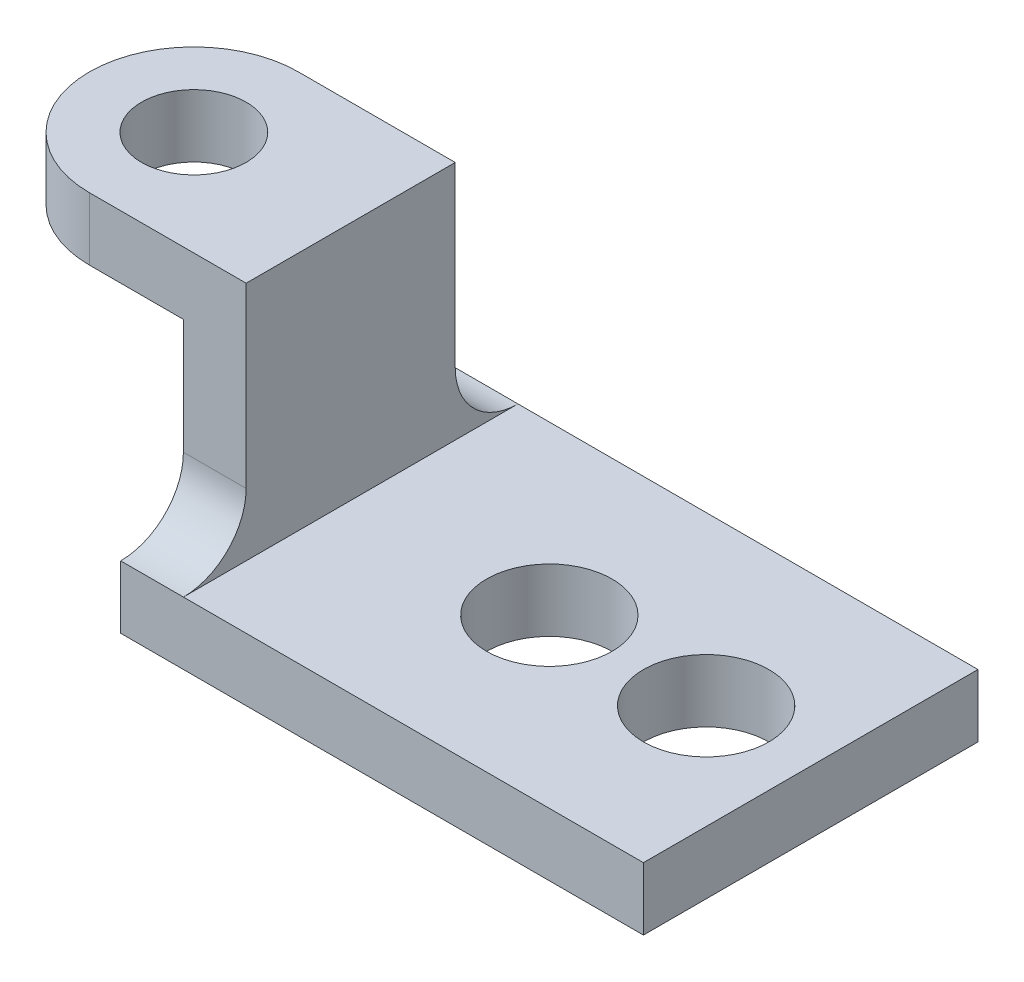
ISO-10303-21;
HEADER;
FILE_DESCRIPTION(('STEP AP214'),'2;1');
FILE_NAME('part.step','',(''),(''),'','','');
FILE_SCHEMA(('AUTOMOTIVE_DESIGN { 1 0 10303 214 1 1 1 1 }'));
ENDSEC;
DATA;
#1=APPLICATION_CONTEXT('core data for automotive mechanical design processes');
#2=APPLICATION_PROTOCOL_DEFINITION('international standard','automotive_design',2000,#1);
#3=PRODUCT_CONTEXT('',#1,'mechanical');
#4=PRODUCT('Part','Part','',(#3));
#5=PRODUCT_RELATED_PRODUCT_CATEGORY('part','',(#4));
#6=PRODUCT_DEFINITION_FORMATION('','',#4);
#7=PRODUCT_DEFINITION_CONTEXT('part definition',#1,'design');
#8=PRODUCT_DEFINITION('design','',#6,#7);
#9=PRODUCT_DEFINITION_SHAPE('','',#8);
#10=(LENGTH_UNIT() NAMED_UNIT(*) SI_UNIT(.MILLI.,.METRE.));
#11=(NAMED_UNIT(*) PLANE_ANGLE_UNIT() SI_UNIT($,.RADIAN.));
#12=(NAMED_UNIT(*) SI_UNIT($,.STERADIAN.) SOLID_ANGLE_UNIT());
#13=UNCERTAINTY_MEASURE_WITH_UNIT(LENGTH_MEASURE(1.E-05),#10,'distance_accuracy_value','');
#14=(GEOMETRIC_REPRESENTATION_CONTEXT(3) GLOBAL_UNCERTAINTY_ASSIGNED_CONTEXT((#13)) GLOBAL_UNIT_ASSIGNED_CONTEXT((#10,
#11,#12)) REPRESENTATION_CONTEXT('',''));
#15=CARTESIAN_POINT('',(0.,0.,0.));
#16=DIRECTION('',(0.,0.,1.));
#17=DIRECTION('',(1.,0.,0.));
#18=AXIS2_PLACEMENT_3D('',#15,#16,#17);
#19=CARTESIAN_POINT('',(-50.,12.,32.));
#20=DIRECTION('',(1.,0.,0.));
#21=DIRECTION('',(0.,0.,-1.));
#22=AXIS2_PLACEMENT_3D('',#19,#20,#21);
#23=PLANE('',#22);
#24=DIRECTION('',(0.,0.,1.));
#25=VECTOR('',#24,1.);
#26=CARTESIAN_POINT('',(-50.,46.,32.));
#27=LINE('',#26,#25);
#28=CARTESIAN_POINT('',(-50.,46.,-20.));
#29=VERTEX_POINT('',#28);
#30=CARTESIAN_POINT('',(-50.,46.,20.));
#31=VERTEX_POINT('',#30);
#32=EDGE_CURVE('E154',#29,#31,#27,.T.);
#33=ORIENTED_EDGE('',*,*,#32,.F.);
#34=DIRECTION('',(0.,-1.,0.));
#35=VECTOR('',#34,1.);
#36=CARTESIAN_POINT('',(-50.,58.,-20.));
#37=LINE('',#36,#35);
#38=CARTESIAN_POINT('',(-50.,24.,-20.));
#39=VERTEX_POINT('',#38);
#40=EDGE_CURVE('E133',#29,#39,#37,.T.);
#41=ORIENTED_EDGE('',*,*,#40,.T.);
#42=CARTESIAN_POINT('',(-50.,24.,-32.));
#43=DIRECTION('',(1.,0.,0.));
#44=DIRECTION('',(0.,0.,-1.));
#45=AXIS2_PLACEMENT_3D('',#42,#43,#44);
#46=CIRCLE('',#45,12.);
#47=CARTESIAN_POINT('',(-50.,12.,-32.));
#48=VERTEX_POINT('',#47);
#49=EDGE_CURVE('E222',#39,#48,#46,.T.);
#50=ORIENTED_EDGE('',*,*,#49,.T.);
#51=DIRECTION('',(0.,-1.,0.));
#52=VECTOR('',#51,1.);
#53=CARTESIAN_POINT('',(-50.,12.,-32.));
#54=LINE('',#53,#52);
#55=CARTESIAN_POINT('',(-50.,0.,-32.));
#56=VERTEX_POINT('',#55);
#57=EDGE_CURVE('E211',#48,#56,#54,.T.);
#58=ORIENTED_EDGE('',*,*,#57,.T.);
#59=DIRECTION('',(0.,0.,1.));
#60=VECTOR('',#59,1.);
#61=CARTESIAN_POINT('',(-50.,0.,32.));
#62=LINE('',#61,#60);
#63=CARTESIAN_POINT('',(-50.,0.,32.));
#64=VERTEX_POINT('',#63);
#65=EDGE_CURVE('E201',#56,#64,#62,.T.);
#66=ORIENTED_EDGE('',*,*,#65,.T.);
#67=DIRECTION('',(0.,-1.,0.));
#68=VECTOR('',#67,1.);
#69=CARTESIAN_POINT('',(-50.,12.,32.));
#70=LINE('',#69,#68);
#71=CARTESIAN_POINT('',(-50.,12.,32.));
#72=VERTEX_POINT('',#71);
#73=EDGE_CURVE('E208',#72,#64,#70,.T.);
#74=ORIENTED_EDGE('',*,*,#73,.F.);
#75=CARTESIAN_POINT('',(-50.,24.,32.));
#76=DIRECTION('',(1.,0.,0.));
#77=DIRECTION('',(0.,0.,-1.));
#78=AXIS2_PLACEMENT_3D('',#75,#76,#77);
#79=CIRCLE('',#78,12.);
#80=CARTESIAN_POINT('',(-50.,24.,20.));
#81=VERTEX_POINT('',#80);
#82=EDGE_CURVE('E11',#72,#81,#79,.T.);
#83=ORIENTED_EDGE('',*,*,#82,.T.);
#84=DIRECTION('',(0.,-1.,0.));
#85=VECTOR('',#84,1.);
#86=CARTESIAN_POINT('',(-50.,58.,20.));
#87=LINE('',#86,#85);
#88=EDGE_CURVE('E175',#31,#81,#87,.T.);
#89=ORIENTED_EDGE('',*,*,#88,.F.);
#90=EDGE_LOOP('',(#33,#41,#50,#58,#66,#74,#83,#89));
#91=FACE_BOUND('',#90,.T.);
#92=ADVANCED_FACE('F39',(#91),#23,.F.);
#93=CARTESIAN_POINT('',(0.,12.,0.));
#94=DIRECTION('',(0.,-1.,0.));
#95=DIRECTION('',(0.,0.,-1.));
#96=AXIS2_PLACEMENT_3D('',#93,#94,#95);
#97=PLANE('',#96);
#98=CARTESIAN_POINT('',(0.,12.,0.));
#99=DIRECTION('',(0.,1.,0.));
#100=DIRECTION('',(0.,0.,1.));
#101=AXIS2_PLACEMENT_3D('',#98,#99,#100);
#102=CIRCLE('',#101,12.);
#103=CARTESIAN_POINT('',(0.,12.,12.));
#104=VERTEX_POINT('',#103);
#105=EDGE_CURVE('E172',#104,#104,#102,.T.);
#106=ORIENTED_EDGE('',*,*,#105,.F.);
#107=EDGE_LOOP('',(#106));
#108=FACE_BOUND('',#107,.T.);
#109=CARTESIAN_POINT('',(30.,12.,0.));
#110=DIRECTION('',(0.,1.,0.));
#111=DIRECTION('',(0.,0.,1.));
#112=AXIS2_PLACEMENT_3D('',#109,#110,#111);
#113=CIRCLE('',#112,12.);
#114=CARTESIAN_POINT('',(30.,12.,12.));
#115=VERTEX_POINT('',#114);
#116=EDGE_CURVE('E182',#115,#115,#113,.T.);
#117=ORIENTED_EDGE('',*,*,#116,.F.);
#118=EDGE_LOOP('',(#117));
#119=FACE_BOUND('',#118,.T.);
#120=DIRECTION('',(-1.,0.,0.));
#121=VECTOR('',#120,1.);
#122=CARTESIAN_POINT('',(-50.,12.,-32.));
#123=LINE('',#122,#121);
#124=CARTESIAN_POINT('',(50.,12.,-32.));
#125=VERTEX_POINT('',#124);
#126=CARTESIAN_POINT('',(-38.,12.,-32.));
#127=VERTEX_POINT('',#126);
#128=EDGE_CURVE('E194',#125,#127,#123,.T.);
#129=ORIENTED_EDGE('',*,*,#128,.T.);
#130=DIRECTION('',(0.,0.,-1.));
#131=VECTOR('',#130,1.);
#132=CARTESIAN_POINT('',(-38.,12.,-20.));
#133=LINE('',#132,#131);
#134=CARTESIAN_POINT('',(-38.,12.,32.));
#135=VERTEX_POINT('',#134);
#136=EDGE_CURVE('E158',#135,#127,#133,.T.);
#137=ORIENTED_EDGE('',*,*,#136,.F.);
#138=DIRECTION('',(1.,0.,0.));
#139=VECTOR('',#138,1.);
#140=CARTESIAN_POINT('',(-50.,12.,32.));
#141=LINE('',#140,#139);
#142=CARTESIAN_POINT('',(50.,12.,32.));
#143=VERTEX_POINT('',#142);
#144=EDGE_CURVE('E193',#135,#143,#141,.T.);
#145=ORIENTED_EDGE('',*,*,#144,.T.);
#146=DIRECTION('',(0.,0.,-1.));
#147=VECTOR('',#146,1.);
#148=CARTESIAN_POINT('',(50.,12.,32.));
#149=LINE('',#148,#147);
#150=EDGE_CURVE('E190',#143,#125,#149,.T.);
#151=ORIENTED_EDGE('',*,*,#150,.T.);
#152=EDGE_LOOP('',(#129,#137,#145,#151));
#153=FACE_BOUND('',#152,.T.);
#154=ADVANCED_FACE('F275',(#108,#119,#153),#97,.F.);
#155=CARTESIAN_POINT('',(0.,0.,0.));
#156=DIRECTION('',(0.,-1.,0.));
#157=DIRECTION('',(0.,0.,-1.));
#158=AXIS2_PLACEMENT_3D('',#155,#156,#157);
#159=PLANE('',#158);
#160=CARTESIAN_POINT('',(30.,0.,0.));
#161=DIRECTION('',(0.,1.,0.));
#162=DIRECTION('',(0.,0.,1.));
#163=AXIS2_PLACEMENT_3D('',#160,#161,#162);
#164=CIRCLE('',#163,12.);
#165=CARTESIAN_POINT('',(30.,0.,12.));
#166=VERTEX_POINT('',#165);
#167=EDGE_CURVE('E180',#166,#166,#164,.T.);
#168=ORIENTED_EDGE('',*,*,#167,.T.);
#169=EDGE_LOOP('',(#168));
#170=FACE_BOUND('',#169,.T.);
#171=DIRECTION('',(0.,0.,-1.));
#172=VECTOR('',#171,1.);
#173=CARTESIAN_POINT('',(50.,0.,32.));
#174=LINE('',#173,#172);
#175=CARTESIAN_POINT('',(50.,0.,32.));
#176=VERTEX_POINT('',#175);
#177=CARTESIAN_POINT('',(50.,0.,-32.));
#178=VERTEX_POINT('',#177);
#179=EDGE_CURVE('E184',#176,#178,#174,.T.);
#180=ORIENTED_EDGE('',*,*,#179,.F.);
#181=DIRECTION('',(1.,0.,0.));
#182=VECTOR('',#181,1.);
#183=CARTESIAN_POINT('',(-50.,0.,32.));
#184=LINE('',#183,#182);
#185=EDGE_CURVE('E192',#64,#176,#184,.T.);
#186=ORIENTED_EDGE('',*,*,#185,.F.);
#187=ORIENTED_EDGE('',*,*,#65,.F.);
#188=DIRECTION('',(-1.,0.,0.));
#189=VECTOR('',#188,1.);
#190=CARTESIAN_POINT('',(-50.,0.,-32.));
#191=LINE('',#190,#189);
#192=EDGE_CURVE('E203',#178,#56,#191,.T.);
#193=ORIENTED_EDGE('',*,*,#192,.F.);
#194=EDGE_LOOP('',(#180,#186,#187,#193));
#195=FACE_BOUND('',#194,.T.);
#196=CARTESIAN_POINT('',(0.,0.,0.));
#197=DIRECTION('',(0.,1.,0.));
#198=DIRECTION('',(0.,0.,1.));
#199=AXIS2_PLACEMENT_3D('',#196,#197,#198);
#200=CIRCLE('',#199,12.);
#201=CARTESIAN_POINT('',(0.,0.,12.));
#202=VERTEX_POINT('',#201);
#203=EDGE_CURVE('E174',#202,#202,#200,.T.);
#204=ORIENTED_EDGE('',*,*,#203,.T.);
#205=EDGE_LOOP('',(#204));
#206=FACE_BOUND('',#205,.T.);
#207=ADVANCED_FACE('F280',(#170,#195,#206),#159,.T.);
#208=CARTESIAN_POINT('',(50.,12.,32.));
#209=DIRECTION('',(-1.,0.,0.));
#210=DIRECTION('',(0.,0.,1.));
#211=AXIS2_PLACEMENT_3D('',#208,#209,#210);
#212=PLANE('',#211);
#213=ORIENTED_EDGE('',*,*,#179,.T.);
#214=DIRECTION('',(0.,-1.,0.));
#215=VECTOR('',#214,1.);
#216=CARTESIAN_POINT('',(50.,12.,-32.));
#217=LINE('',#216,#215);
#218=EDGE_CURVE('E212',#125,#178,#217,.T.);
#219=ORIENTED_EDGE('',*,*,#218,.F.);
#220=ORIENTED_EDGE('',*,*,#150,.F.);
#221=DIRECTION('',(0.,-1.,0.));
#222=VECTOR('',#221,1.);
#223=CARTESIAN_POINT('',(50.,12.,32.));
#224=LINE('',#223,#222);
#225=EDGE_CURVE('E196',#143,#176,#224,.T.);
#226=ORIENTED_EDGE('',*,*,#225,.T.);
#227=EDGE_LOOP('',(#213,#219,#220,#226));
#228=FACE_BOUND('',#227,.T.);
#229=ADVANCED_FACE('F282',(#228),#212,.F.);
#230=CARTESIAN_POINT('',(-50.,12.,-32.));
#231=DIRECTION('',(0.,0.,1.));
#232=DIRECTION('',(1.,0.,0.));
#233=AXIS2_PLACEMENT_3D('',#230,#231,#232);
#234=PLANE('',#233);
#235=ORIENTED_EDGE('',*,*,#192,.T.);
#236=ORIENTED_EDGE('',*,*,#57,.F.);
#237=EDGE_CURVE('E187',#127,#48,#123,.T.);
#238=ORIENTED_EDGE('',*,*,#237,.F.);
#239=ORIENTED_EDGE('',*,*,#128,.F.);
#240=ORIENTED_EDGE('',*,*,#218,.T.);
#241=EDGE_LOOP('',(#235,#236,#238,#239,#240));
#242=FACE_BOUND('',#241,.T.);
#243=ADVANCED_FACE('F244',(#242),#234,.F.);
#244=CARTESIAN_POINT('',(-50.,12.,32.));
#245=DIRECTION('',(0.,0.,-1.));
#246=DIRECTION('',(-1.,0.,0.));
#247=AXIS2_PLACEMENT_3D('',#244,#245,#246);
#248=PLANE('',#247);
#249=ORIENTED_EDGE('',*,*,#185,.T.);
#250=ORIENTED_EDGE('',*,*,#225,.F.);
#251=ORIENTED_EDGE('',*,*,#144,.F.);
#252=EDGE_CURVE('E198',#72,#135,#141,.T.);
#253=ORIENTED_EDGE('',*,*,#252,.F.);
#254=ORIENTED_EDGE('',*,*,#73,.T.);
#255=EDGE_LOOP('',(#249,#250,#251,#253,#254));
#256=FACE_BOUND('',#255,.T.);
#257=ADVANCED_FACE('F235',(#256),#248,.F.);
#258=CARTESIAN_POINT('',(30.,12.,0.));
#259=DIRECTION('',(0.,-1.,0.));
#260=DIRECTION('',(0.,0.,-1.));
#261=AXIS2_PLACEMENT_3D('',#258,#259,#260);
#262=CYLINDRICAL_SURFACE('',#261,12.);
#263=ORIENTED_EDGE('',*,*,#116,.T.);
#264=EDGE_LOOP('',(#263));
#265=FACE_BOUND('',#264,.T.);
#266=ORIENTED_EDGE('',*,*,#167,.F.);
#267=EDGE_LOOP('',(#266));
#268=FACE_BOUND('',#267,.T.);
#269=ADVANCED_FACE('F304',(#265,#268),#262,.F.);
#270=CARTESIAN_POINT('',(0.,12.,0.));
#271=DIRECTION('',(0.,-1.,0.));
#272=DIRECTION('',(0.,0.,-1.));
#273=AXIS2_PLACEMENT_3D('',#270,#271,#272);
#274=CYLINDRICAL_SURFACE('',#273,12.);
#275=ORIENTED_EDGE('',*,*,#105,.T.);
#276=EDGE_LOOP('',(#275));
#277=FACE_BOUND('',#276,.T.);
#278=ORIENTED_EDGE('',*,*,#203,.F.);
#279=EDGE_LOOP('',(#278));
#280=FACE_BOUND('',#279,.T.);
#281=ADVANCED_FACE('F297',(#277,#280),#274,.F.);
#282=CARTESIAN_POINT('',(-50.,58.,20.));
#283=DIRECTION('',(0.,0.,-1.));
#284=DIRECTION('',(-1.,0.,0.));
#285=AXIS2_PLACEMENT_3D('',#282,#283,#284);
#286=PLANE('',#285);
#287=ORIENTED_EDGE('',*,*,#88,.T.);
#288=DIRECTION('',(1.,0.,0.));
#289=VECTOR('',#288,1.);
#290=CARTESIAN_POINT('',(-38.,24.,20.));
#291=LINE('',#290,#289);
#292=CARTESIAN_POINT('',(-38.,24.,20.));
#293=VERTEX_POINT('',#292);
#294=EDGE_CURVE('E218',#81,#293,#291,.T.);
#295=ORIENTED_EDGE('',*,*,#294,.T.);
#296=DIRECTION('',(0.,-1.,0.));
#297=VECTOR('',#296,1.);
#298=CARTESIAN_POINT('',(-38.,58.,20.));
#299=LINE('',#298,#297);
#300=CARTESIAN_POINT('',(-38.,58.,20.));
#301=VERTEX_POINT('',#300);
#302=EDGE_CURVE('E166',#301,#293,#299,.T.);
#303=ORIENTED_EDGE('',*,*,#302,.F.);
#304=DIRECTION('',(1.,0.,0.));
#305=VECTOR('',#304,1.);
#306=CARTESIAN_POINT('',(-50.,58.,20.));
#307=LINE('',#306,#305);
#308=CARTESIAN_POINT('',(-68.,58.,20.));
#309=VERTEX_POINT('',#308);
#310=EDGE_CURVE('E157',#309,#301,#307,.T.);
#311=ORIENTED_EDGE('',*,*,#310,.F.);
#312=DIRECTION('',(0.,1.,0.));
#313=VECTOR('',#312,1.);
#314=CARTESIAN_POINT('',(-68.,46.,20.));
#315=LINE('',#314,#313);
#316=CARTESIAN_POINT('',(-68.,46.,20.));
#317=VERTEX_POINT('',#316);
#318=EDGE_CURVE('E141',#317,#309,#315,.T.);
#319=ORIENTED_EDGE('',*,*,#318,.F.);
#320=DIRECTION('',(1.,0.,0.));
#321=VECTOR('',#320,1.);
#322=CARTESIAN_POINT('',(-68.,46.,20.));
#323=LINE('',#322,#321);
#324=EDGE_CURVE('E145',#317,#31,#323,.T.);
#325=ORIENTED_EDGE('',*,*,#324,.T.);
#326=EDGE_LOOP('',(#287,#295,#303,#311,#319,#325));
#327=FACE_BOUND('',#326,.T.);
#328=ADVANCED_FACE('F240',(#327),#286,.F.);
#329=CARTESIAN_POINT('',(-38.,58.,-20.));
#330=DIRECTION('',(-1.,0.,0.));
#331=DIRECTION('',(0.,0.,1.));
#332=AXIS2_PLACEMENT_3D('',#329,#330,#331);
#333=PLANE('',#332);
#334=ORIENTED_EDGE('',*,*,#302,.T.);
#335=CARTESIAN_POINT('',(-38.,24.,32.));
#336=DIRECTION('',(-1.,0.,0.));
#337=DIRECTION('',(0.,0.,1.));
#338=AXIS2_PLACEMENT_3D('',#335,#336,#337);
#339=CIRCLE('',#338,12.);
#340=EDGE_CURVE('E50',#293,#135,#339,.T.);
#341=ORIENTED_EDGE('',*,*,#340,.T.);
#342=ORIENTED_EDGE('',*,*,#136,.T.);
#343=CARTESIAN_POINT('',(-38.,24.,-32.));
#344=DIRECTION('',(-1.,0.,0.));
#345=DIRECTION('',(0.,0.,1.));
#346=AXIS2_PLACEMENT_3D('',#343,#344,#345);
#347=CIRCLE('',#346,12.);
#348=CARTESIAN_POINT('',(-38.,24.,-20.));
#349=VERTEX_POINT('',#348);
#350=EDGE_CURVE('E224',#127,#349,#347,.T.);
#351=ORIENTED_EDGE('',*,*,#350,.T.);
#352=DIRECTION('',(0.,-1.,0.));
#353=VECTOR('',#352,1.);
#354=CARTESIAN_POINT('',(-38.,58.,-20.));
#355=LINE('',#354,#353);
#356=CARTESIAN_POINT('',(-38.,58.,-20.));
#357=VERTEX_POINT('',#356);
#358=EDGE_CURVE('E170',#357,#349,#355,.T.);
#359=ORIENTED_EDGE('',*,*,#358,.F.);
#360=DIRECTION('',(0.,0.,-1.));
#361=VECTOR('',#360,1.);
#362=CARTESIAN_POINT('',(-38.,58.,-20.));
#363=LINE('',#362,#361);
#364=EDGE_CURVE('E161',#301,#357,#363,.T.);
#365=ORIENTED_EDGE('',*,*,#364,.F.);
#366=EDGE_LOOP('',(#334,#341,#342,#351,#359,#365));
#367=FACE_BOUND('',#366,.T.);
#368=ADVANCED_FACE('F228',(#367),#333,.F.);
#369=CARTESIAN_POINT('',(-50.,58.,-20.));
#370=DIRECTION('',(0.,0.,1.));
#371=DIRECTION('',(1.,0.,0.));
#372=AXIS2_PLACEMENT_3D('',#369,#370,#371);
#373=PLANE('',#372);
#374=ORIENTED_EDGE('',*,*,#358,.T.);
#375=DIRECTION('',(-1.,0.,0.));
#376=VECTOR('',#375,1.);
#377=CARTESIAN_POINT('',(-50.,24.,-20.));
#378=LINE('',#377,#376);
#379=EDGE_CURVE('E220',#349,#39,#378,.T.);
#380=ORIENTED_EDGE('',*,*,#379,.T.);
#381=ORIENTED_EDGE('',*,*,#40,.F.);
#382=DIRECTION('',(-1.,0.,0.));
#383=VECTOR('',#382,1.);
#384=CARTESIAN_POINT('',(-38.,46.,-20.));
#385=LINE('',#384,#383);
#386=CARTESIAN_POINT('',(-68.,46.,-20.));
#387=VERTEX_POINT('',#386);
#388=EDGE_CURVE('E124',#29,#387,#385,.T.);
#389=ORIENTED_EDGE('',*,*,#388,.T.);
#390=DIRECTION('',(0.,1.,0.));
#391=VECTOR('',#390,1.);
#392=CARTESIAN_POINT('',(-68.,46.,-20.));
#393=LINE('',#392,#391);
#394=CARTESIAN_POINT('',(-68.,58.,-20.));
#395=VERTEX_POINT('',#394);
#396=EDGE_CURVE('E130',#387,#395,#393,.T.);
#397=ORIENTED_EDGE('',*,*,#396,.T.);
#398=DIRECTION('',(-1.,0.,0.));
#399=VECTOR('',#398,1.);
#400=CARTESIAN_POINT('',(-50.,58.,-20.));
#401=LINE('',#400,#399);
#402=EDGE_CURVE('E162',#357,#395,#401,.T.);
#403=ORIENTED_EDGE('',*,*,#402,.F.);
#404=EDGE_LOOP('',(#374,#380,#381,#389,#397,#403));
#405=FACE_BOUND('',#404,.T.);
#406=ADVANCED_FACE('F123',(#405),#373,.F.);
#407=CARTESIAN_POINT('',(0.,58.,0.));
#408=DIRECTION('',(0.,1.,0.));
#409=DIRECTION('',(0.,0.,1.));
#410=AXIS2_PLACEMENT_3D('',#407,#408,#409);
#411=PLANE('',#410);
#412=ORIENTED_EDGE('',*,*,#402,.T.);
#413=CARTESIAN_POINT('',(-68.,58.,0.));
#414=DIRECTION('',(0.,1.,0.));
#415=DIRECTION('',(0.,0.,1.));
#416=AXIS2_PLACEMENT_3D('',#413,#414,#415);
#417=CIRCLE('',#416,20.);
#418=EDGE_CURVE('E137',#395,#309,#417,.T.);
#419=ORIENTED_EDGE('',*,*,#418,.T.);
#420=ORIENTED_EDGE('',*,*,#310,.T.);
#421=ORIENTED_EDGE('',*,*,#364,.T.);
#422=EDGE_LOOP('',(#412,#419,#420,#421));
#423=FACE_BOUND('',#422,.T.);
#424=CARTESIAN_POINT('',(-68.,58.,0.));
#425=DIRECTION('',(0.,1.,0.));
#426=DIRECTION('',(0.,0.,1.));
#427=AXIS2_PLACEMENT_3D('',#424,#425,#426);
#428=CIRCLE('',#427,10.);
#429=CARTESIAN_POINT('',(-68.,58.,10.));
#430=VERTEX_POINT('',#429);
#431=EDGE_CURVE('E254',#430,#430,#428,.T.);
#432=ORIENTED_EDGE('',*,*,#431,.F.);
#433=EDGE_LOOP('',(#432));
#434=FACE_BOUND('',#433,.T.);
#435=ADVANCED_FACE('F246',(#423,#434),#411,.T.);
#436=CARTESIAN_POINT('',(-68.,46.,0.));
#437=DIRECTION('',(0.,1.,0.));
#438=DIRECTION('',(0.,0.,1.));
#439=AXIS2_PLACEMENT_3D('',#436,#437,#438);
#440=PLANE('',#439);
#441=CARTESIAN_POINT('',(-68.,46.,0.));
#442=DIRECTION('',(0.,1.,0.));
#443=DIRECTION('',(0.,0.,1.));
#444=AXIS2_PLACEMENT_3D('',#441,#442,#443);
#445=CIRCLE('',#444,10.);
#446=CARTESIAN_POINT('',(-68.,46.,10.));
#447=VERTEX_POINT('',#446);
#448=EDGE_CURVE('E152',#447,#447,#445,.T.);
#449=ORIENTED_EDGE('',*,*,#448,.T.);
#450=EDGE_LOOP('',(#449));
#451=FACE_BOUND('',#450,.T.);
#452=ORIENTED_EDGE('',*,*,#388,.F.);
#453=ORIENTED_EDGE('',*,*,#32,.T.);
#454=ORIENTED_EDGE('',*,*,#324,.F.);
#455=CARTESIAN_POINT('',(-68.,46.,0.));
#456=DIRECTION('',(0.,1.,0.));
#457=DIRECTION('',(0.,0.,1.));
#458=AXIS2_PLACEMENT_3D('',#455,#456,#457);
#459=CIRCLE('',#458,20.);
#460=EDGE_CURVE('E132',#387,#317,#459,.T.);
#461=ORIENTED_EDGE('',*,*,#460,.F.);
#462=EDGE_LOOP('',(#452,#453,#454,#461));
#463=FACE_BOUND('',#462,.T.);
#464=ADVANCED_FACE('F150',(#451,#463),#440,.F.);
#465=CARTESIAN_POINT('',(-68.,46.,0.));
#466=DIRECTION('',(0.,1.,0.));
#467=DIRECTION('',(0.,0.,1.));
#468=AXIS2_PLACEMENT_3D('',#465,#466,#467);
#469=CYLINDRICAL_SURFACE('',#468,20.);
#470=ORIENTED_EDGE('',*,*,#418,.F.);
#471=ORIENTED_EDGE('',*,*,#396,.F.);
#472=ORIENTED_EDGE('',*,*,#460,.T.);
#473=ORIENTED_EDGE('',*,*,#318,.T.);
#474=EDGE_LOOP('',(#470,#471,#472,#473));
#475=FACE_BOUND('',#474,.T.);
#476=ADVANCED_FACE('F138',(#475),#469,.T.);
#477=CARTESIAN_POINT('',(-68.,46.,0.));
#478=DIRECTION('',(0.,1.,0.));
#479=DIRECTION('',(0.,0.,1.));
#480=AXIS2_PLACEMENT_3D('',#477,#478,#479);
#481=CYLINDRICAL_SURFACE('',#480,10.);
#482=ORIENTED_EDGE('',*,*,#448,.F.);
#483=EDGE_LOOP('',(#482));
#484=FACE_BOUND('',#483,.T.);
#485=ORIENTED_EDGE('',*,*,#431,.T.);
#486=EDGE_LOOP('',(#485));
#487=FACE_BOUND('',#486,.T.);
#488=ADVANCED_FACE('F265',(#484,#487),#481,.F.);
#489=CARTESIAN_POINT('',(-50.,24.,-32.));
#490=DIRECTION('',(1.,0.,0.));
#491=DIRECTION('',(0.,0.,-1.));
#492=AXIS2_PLACEMENT_3D('',#489,#490,#491);
#493=CYLINDRICAL_SURFACE('',#492,12.);
#494=ORIENTED_EDGE('',*,*,#350,.F.);
#495=ORIENTED_EDGE('',*,*,#237,.T.);
#496=ORIENTED_EDGE('',*,*,#49,.F.);
#497=ORIENTED_EDGE('',*,*,#379,.F.);
#498=EDGE_LOOP('',(#494,#495,#496,#497));
#499=FACE_BOUND('',#498,.T.);
#500=ADVANCED_FACE('F247',(#499),#493,.F.);
#501=CARTESIAN_POINT('',(-50.,24.,32.));
#502=DIRECTION('',(-1.,0.,0.));
#503=DIRECTION('',(0.,0.,1.));
#504=AXIS2_PLACEMENT_3D('',#501,#502,#503);
#505=CYLINDRICAL_SURFACE('',#504,12.);
#506=ORIENTED_EDGE('',*,*,#82,.F.);
#507=ORIENTED_EDGE('',*,*,#252,.T.);
#508=ORIENTED_EDGE('',*,*,#340,.F.);
#509=ORIENTED_EDGE('',*,*,#294,.F.);
#510=EDGE_LOOP('',(#506,#507,#508,#509));
#511=FACE_BOUND('',#510,.T.);
#512=ADVANCED_FACE('F41',(#511),#505,.F.);
#513=CLOSED_SHELL('',(#92,#154,#207,#229,#243,#257,#269,#281,#328,#368,#406,#435,#464,#476,#488,
#500,#512));
#514=MANIFOLD_SOLID_BREP('B2',#513);
#515=ADVANCED_BREP_SHAPE_REPRESENTATION('',(#18,#514),#14);
#516=SHAPE_DEFINITION_REPRESENTATION(#9,#515);
ENDSEC;
END-ISO-10303-21;
